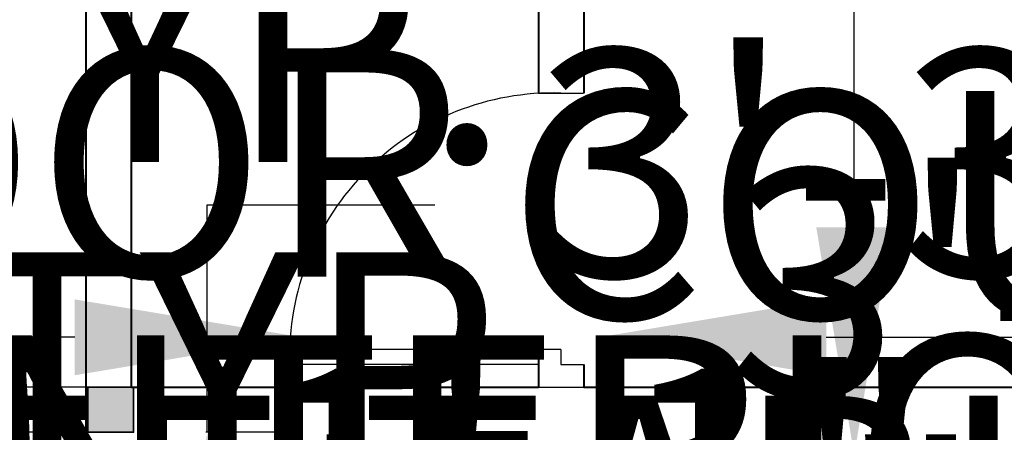
# Model space of a CAD drawing. Units: inches. Extents: x 7323 to 9737, y 2037 to 3322.
# Tile 11 of 19: x 8999 to 9130, y 2513 to 2568. Entities that reach past the tile are written whole.
import ezdxf

# ---------------------------------------------------------------- set-up
doc = ezdxf.new("R2010")
doc.units = ezdxf.units.IN
doc.header["$MEASUREMENT"] = 0
for name, color, linetype, lineweight in [('A-ANNO-DIMS', 2, 'Continuous', 18), ('A-COLS', 1, 'Continuous', 35), ('A-DOOR', 4, 'Continuous', 25), ('A-WALL', 7, 'Continuous', 40)]:
    doc.layers.add(name, color=color, linetype=linetype, lineweight=lineweight)
doc.layers.add('A-COLS-PATT', color=18, linetype='Continuous', lineweight=13, true_color=0x000000)
doc.styles.get("Standard").update_dxf_attribs({"font": 'arial.ttf'})
doc.dimstyles.get("Standard").update_dxf_attribs({"dimtxt": 30.18, "dimasz": 30.18, "dimexe": 0.18, "dimexo": 0.0625, "dimgap": 0.09, "dimtad": 0, "dimtih": 1, "dimtoh": 1, "dimdec": 0, "dimzin": 0, "dimdsep": 46, "dimlunit": 3, "dimtxsty": 'Standard', "dimcen": 0.09, "dimadec": 0, "dimazin": 0, "dimtfac": 1, "dimtdec": 0, "dimtofl": 0, "dimtmove": 0, "dimatfit": 3, "dimfxl": 1, "dimtolj": 1, "dimtzin": 0, "dimarcsym": 0})

# ---------------------------------------------------------------- blocks, each defined once
blk = doc.blocks.new('*D11')
at = {"layer": 'A-ANNO-DIMS', "color": 0, "lineweight": -2, "transparency": 16777216}
for p, q in [((9007.88, 2687.3), (8985.8, 2687.3)), ((8985.98, 2657.12), (8985.98, 2458.79)), ((8985.98, 2229.48), (8985.98, 2427.8)), ((9007.88, 2199.3), (8985.8, 2199.3))]:
    blk.add_line(p, q, dxfattribs=at)
at = {"layer": 'A-ANNO-DIMS', "color": 0, "transparency": 16777216}
for points in [[(8980.95, 2657.12), (8991.01, 2657.12), (8985.98, 2687.3)], [(8980.95, 2229.48), (8991.01, 2229.48), (8985.98, 2199.3)]]:
    blk.add_solid(points, dxfattribs=at)
at = {"layer": 'Defpoints', "color": 0, "transparency": 16777216}
for p in [(9007.95, 2687.3), (8985.98, 2199.3), (9007.95, 2199.3)]:
    blk.add_point(p, dxfattribs=at)
at = {"layer": 'A-ANNO-DIMS', "color": 0, "transparency": 16777216, "insert": (8985.98, 2443.3), "char_height": 30.18, "attachment_point": 5}
blk.add_mtext('\\A1;40\'-8"', dxfattribs=at)
blk = doc.blocks.new('DOOR-36')
for p, q in [((33.01, 39), (39.01, 39)), ((36.01, 5), (0.01, 5)), ((36.01, 5), (36.01, 3)), ((33.01, 3), (0.01, 3)), ((36.01, 3), (39.01, 3)), ((33.01, 0), (39.01, 0))]:
    blk.add_line(p, q)
blk.add_arc((35.01, 4), 35.01, 88.3634, 181.6366)
blk = doc.blocks.new('COL-PLAN-6IN')
blk.add_lwpolyline([(0, 6), (0, 6), (6.06, 6), (6.06, 6), (6.06, 0), (6.06, 0), (0, 0), (0, 0)], close=True)
blk = doc.blocks.new('*D37')
at = {"layer": 'A-ANNO-DIMS', "color": 0, "lineweight": -2, "transparency": 16777216}
for p, q in [((9279.75, 2656.48), (9279.75, 2686.66)), ((9272.01, 2626.3), (9279.93, 2626.3)), ((9272.01, 2574.3), (9279.93, 2574.3)), ((9279.75, 2544.12), (9279.75, 2513.94))]:
    blk.add_line(p, q, dxfattribs=at)
at = {"layer": 'A-ANNO-DIMS', "color": 0, "transparency": 16777216}
for points in [[(9274.72, 2656.48), (9284.78, 2656.48), (9279.75, 2626.3)], [(9274.72, 2544.12), (9284.78, 2544.12), (9279.75, 2574.3)]]:
    blk.add_solid(points, dxfattribs=at)
at = {"layer": 'Defpoints', "color": 0, "transparency": 16777216}
for p in [(9271.95, 2626.3), (9271.95, 2574.3), (9279.75, 2574.3)]:
    blk.add_point(p, dxfattribs=at)
at = {"layer": 'A-ANNO-DIMS', "color": 0, "transparency": 16777216, "insert": (9279.75, 2600.3), "char_height": 30.18, "attachment_point": 5}
blk.add_mtext('\\A1;WINDOW 4\'-4" TYP.', dxfattribs=at)
blk = doc.blocks.new('*D39')
at = {"layer": 'A-ANNO-DIMS', "color": 0, "lineweight": -2, "transparency": 16777216}
for p, q in [((8647.94, 2549.03), (8617.76, 2549.03)), ((8678.12, 2543.2), (8678.12, 2549.21)), ((8717.39, 2543.2), (8717.39, 2549.21)), ((8747.57, 2549.03), (8777.75, 2549.03))]:
    blk.add_line(p, q, dxfattribs=at)
at = {"layer": 'A-ANNO-DIMS', "color": 0, "transparency": 16777216}
for points in [[(8647.94, 2554.06), (8647.94, 2544), (8678.12, 2549.03)], [(8747.57, 2554.06), (8747.57, 2544), (8717.39, 2549.03)]]:
    blk.add_solid(points, dxfattribs=at)
at = {"layer": 'Defpoints', "color": 0, "transparency": 16777216}
for p in [(8717.39, 2549.03), (8678.12, 2543.14), (8717.39, 2543.14)]:
    blk.add_point(p, dxfattribs=at)
at = {"layer": 'A-ANNO-DIMS', "color": 0, "transparency": 16777216, "insert": (9057.19, 2549.03), "char_height": 30.18, "attachment_point": 5}
blk.add_mtext('\\A1;SINGLE DOOR 3\'-3 1/2" TYP.', dxfattribs=at)
blk = doc.blocks.new('*D41')
at = {"layer": 'A-ANNO-DIMS', "color": 0, "lineweight": -2, "transparency": 16777216}
for p, q in [((8661.59, 2428.04), (8661.59, 2458.22)), ((8661.59, 2458.22), (8691.77, 2458.22)), ((8657.46, 2397.86), (8661.77, 2397.86)), ((8657.46, 2369.86), (8661.77, 2369.86)), ((8661.59, 2339.68), (8661.59, 2309.5))]:
    blk.add_line(p, q, dxfattribs=at)
at = {"layer": 'A-ANNO-DIMS', "color": 0, "transparency": 16777216}
for points in [[(8656.56, 2428.04), (8666.62, 2428.04), (8661.59, 2397.86)], [(8656.56, 2339.68), (8666.62, 2339.68), (8661.59, 2369.86)]]:
    blk.add_solid(points, dxfattribs=at)
at = {"layer": 'Defpoints', "color": 0, "transparency": 16777216}
for p in [(8657.39, 2397.86), (8661.59, 2397.86), (8657.39, 2369.86)]:
    blk.add_point(p, dxfattribs=at)
at = {"layer": 'A-ANNO-DIMS', "color": 0, "transparency": 16777216, "insert": (8945.06, 2458.22), "char_height": 30.18, "attachment_point": 5}
blk.add_mtext('\\A1;VENT WINDOW 2\'-4" TYP.', dxfattribs=at)
blk = doc.blocks.new('*D47')
at = {"layer": 'A-ANNO-DIMS', "color": 0, "lineweight": -2, "transparency": 16777216}
for p, q in [((8839.73, 2461.79), (8839.73, 2464.67)), ((8858.14, 2461.79), (8858.14, 2464.67)), ((8809.55, 2464.49), (8779.37, 2464.49)), ((8888.32, 2464.49), (8918.5, 2464.49))]:
    blk.add_line(p, q, dxfattribs=at)
at = {"layer": 'A-ANNO-DIMS', "color": 0, "transparency": 16777216}
for points in [[(8809.55, 2469.52), (8809.55, 2459.46), (8839.73, 2464.49)], [(8888.32, 2469.52), (8888.32, 2459.46), (8858.14, 2464.49)]]:
    blk.add_solid(points, dxfattribs=at)
at = {"layer": 'Defpoints', "color": 0, "transparency": 16777216}
for p in [(8858.14, 2464.49), (8839.73, 2461.73), (8858.14, 2461.73)]:
    blk.add_point(p, dxfattribs=at)
at = {"layer": 'A-ANNO-DIMS', "color": 0, "transparency": 16777216, "insert": (9164.9, 2464.49), "char_height": 30.18, "attachment_point": 5}
blk.add_mtext('\\A1;ARMCHAIR 1\'-6 1/2" TYP.', dxfattribs=at)
blk = doc.blocks.new('*D48')
at = {"layer": 'A-ANNO-DIMS', "color": 0, "lineweight": -2, "transparency": 16777216}
for p, q in [((8836.96, 2491.91), (8836.96, 2522.09)), ((8836.96, 2522.09), (8867.14, 2522.09)), ((8839.66, 2461.73), (8836.78, 2461.73)), ((8839.66, 2451.75), (8836.78, 2451.75)), ((8836.96, 2421.57), (8836.96, 2391.39))]:
    blk.add_line(p, q, dxfattribs=at)
at = {"layer": 'A-ANNO-DIMS', "color": 0, "transparency": 16777216}
for points in [[(8831.93, 2491.91), (8841.99, 2491.91), (8836.96, 2461.73)], [(8831.93, 2421.57), (8841.99, 2421.57), (8836.96, 2451.75)]]:
    blk.add_solid(points, dxfattribs=at)
at = {"layer": 'Defpoints', "color": 0, "transparency": 16777216}
for p in [(8836.96, 2461.73), (8839.73, 2461.73), (8839.73, 2451.75)]:
    blk.add_point(p, dxfattribs=at)
at = {"layer": 'A-ANNO-DIMS', "color": 0, "transparency": 16777216, "insert": (8970.94, 2522.09), "char_height": 30.18, "attachment_point": 5}
blk.add_mtext('\\A1;0\'-10" TYP.', dxfattribs=at)
blk = doc.blocks.new('*D52')
at = {"layer": 'A-ANNO-DIMS', "color": 0, "lineweight": -2, "transparency": 16777216}
for p, q in [((9220.65, 2583.03), (9220.65, 2613.21)), ((9209.01, 2552.85), (9220.83, 2552.85)), ((9209.01, 2513.3), (9220.83, 2513.3)), ((9220.65, 2483.12), (9220.65, 2452.94))]:
    blk.add_line(p, q, dxfattribs=at)
at = {"layer": 'A-ANNO-DIMS', "color": 0, "transparency": 16777216}
for points in [[(9215.62, 2583.03), (9225.68, 2583.03), (9220.65, 2552.85)], [(9215.62, 2483.12), (9225.68, 2483.12), (9220.65, 2513.3)]]:
    blk.add_solid(points, dxfattribs=at)
at = {"layer": 'Defpoints', "color": 0, "transparency": 16777216}
for p in [(9208.95, 2552.85), (9220.65, 2552.85), (9208.95, 2513.3)]:
    blk.add_point(p, dxfattribs=at)
at = {"layer": 'A-ANNO-DIMS', "color": 0, "transparency": 16777216, "insert": (9220.65, 2533.07), "char_height": 30.18, "attachment_point": 5}
blk.add_mtext('\\A1;3\'-3 1/2" TYP.', dxfattribs=at)
blk = doc.blocks.new('*D53')
at = {"layer": 'A-ANNO-DIMS', "color": 0, "lineweight": -2, "transparency": 16777216}
for p, q in [((8826.85, 2511.06), (8796.67, 2511.06)), ((8857.03, 2503.93), (8857.03, 2511.24)), ((8905.03, 2503.93), (8905.03, 2511.24)), ((8935.21, 2511.06), (8965.39, 2511.06))]:
    blk.add_line(p, q, dxfattribs=at)
at = {"layer": 'A-ANNO-DIMS', "color": 0, "transparency": 16777216}
for points in [[(8826.85, 2516.09), (8826.85, 2506.03), (8857.03, 2511.06)], [(8935.21, 2516.09), (8935.21, 2506.03), (8905.03, 2511.06)]]:
    blk.add_solid(points, dxfattribs=at)
at = {"layer": 'Defpoints', "color": 0, "transparency": 16777216}
for p in [(8905.03, 2511.06), (8857.03, 2503.86), (8905.03, 2503.86)]:
    blk.add_point(p, dxfattribs=at)
at = {"layer": 'A-ANNO-DIMS', "color": 0, "transparency": 16777216, "insert": (9261.3, 2511.06), "char_height": 30.18, "attachment_point": 5}
blk.add_mtext('\\A1;INTERIOR WINDOW 4\'-0" TYP.', dxfattribs=at)
blk = doc.blocks.new('*D54')
at = {"layer": 'A-ANNO-DIMS', "color": 0, "lineweight": -2, "transparency": 16777216}
for p, q in [((8849.83, 2534.04), (8849.83, 2564.22)), ((8849.83, 2564.22), (8880.01, 2564.22)), ((8856.96, 2503.86), (8849.65, 2503.86)), ((8856.96, 2497.86), (8849.65, 2497.86)), ((8849.83, 2467.68), (8849.83, 2437.5))]:
    blk.add_line(p, q, dxfattribs=at)
at = {"layer": 'A-ANNO-DIMS', "color": 0, "transparency": 16777216}
for points in [[(8844.8, 2534.04), (8854.86, 2534.04), (8849.83, 2503.86)], [(8844.8, 2467.68), (8854.86, 2467.68), (8849.83, 2497.86)]]:
    blk.add_solid(points, dxfattribs=at)
at = {"layer": 'Defpoints', "color": 0, "transparency": 16777216}
for p in [(8849.83, 2503.86), (8857.03, 2503.86), (8857.03, 2497.86)]:
    blk.add_point(p, dxfattribs=at)
at = {"layer": 'A-ANNO-DIMS', "color": 0, "transparency": 16777216, "insert": (8972.08, 2564.22), "char_height": 30.18, "attachment_point": 5}
blk.add_mtext('\\A1;0\'-6" TYP.', dxfattribs=at)
blk = doc.blocks.new('*D59')
at = {"layer": 'A-ANNO-DIMS', "color": 0, "lineweight": -2, "transparency": 16777216}
for p, q in [((9064.67, 2473.96), (9064.67, 2467.95)), ((9103.95, 2473.96), (9103.95, 2467.95)), ((9034.49, 2468.13), (9004.31, 2468.13)), ((9134.13, 2468.13), (9164.31, 2468.13))]:
    blk.add_line(p, q, dxfattribs=at)
at = {"layer": 'A-ANNO-DIMS', "color": 0, "transparency": 16777216}
for points in [[(9034.49, 2473.16), (9034.49, 2463.1), (9064.67, 2468.13)], [(9134.13, 2473.16), (9134.13, 2463.1), (9103.95, 2468.13)]]:
    blk.add_solid(points, dxfattribs=at)
at = {"layer": 'Defpoints', "color": 0, "transparency": 16777216}
for p in [(9064.67, 2474.02), (9103.95, 2474.02), (9103.95, 2468.13)]:
    blk.add_point(p, dxfattribs=at)
at = {"layer": 'A-ANNO-DIMS', "color": 0, "transparency": 16777216, "insert": (9458.35, 2468.13), "char_height": 30.18, "attachment_point": 5}
blk.add_mtext('\\A1;KITCHEN DOOR 3\'-3 1/2" TYP.', dxfattribs=at)
blk = doc.blocks.new('*D60')
at = {"layer": 'A-ANNO-DIMS', "color": 0, "lineweight": -2, "transparency": 16777216}
for p, q in [((9109.84, 2540.48), (9109.84, 2570.66)), ((9104.01, 2510.3), (9110.02, 2510.3)), ((9104.01, 2474.02), (9110.02, 2474.02)), ((9109.84, 2443.84), (9109.84, 2413.66))]:
    blk.add_line(p, q, dxfattribs=at)
at = {"layer": 'A-ANNO-DIMS', "color": 0, "transparency": 16777216}
for points in [[(9104.81, 2540.48), (9114.87, 2540.48), (9109.84, 2510.3)], [(9104.81, 2443.84), (9114.87, 2443.84), (9109.84, 2474.02)]]:
    blk.add_solid(points, dxfattribs=at)
at = {"layer": 'Defpoints', "color": 0, "transparency": 16777216}
for p in [(9103.95, 2510.3), (9109.84, 2510.3), (9103.95, 2474.02)]:
    blk.add_point(p, dxfattribs=at)
at = {"layer": 'A-ANNO-DIMS', "color": 0, "transparency": 16777216, "insert": (9109.84, 2492.16), "char_height": 30.18, "attachment_point": 5}
blk.add_mtext('\\A1;3\'-0 1/2" TYP.', dxfattribs=at)
blk = doc.blocks.new('*D63')
at = {"layer": 'A-ANNO-DIMS', "color": 0, "lineweight": -2, "transparency": 16777216}
for p, q in [((8744.72, 2466.22), (8744.72, 2496.4)), ((8744.72, 2496.4), (8774.9, 2496.4)), ((8741.46, 2436.04), (8744.9, 2436.04)), ((8741.46, 2413.86), (8744.9, 2413.86)), ((8744.72, 2383.68), (8744.72, 2353.5))]:
    blk.add_line(p, q, dxfattribs=at)
at = {"layer": 'A-ANNO-DIMS', "color": 0, "transparency": 16777216}
for points in [[(8739.69, 2466.22), (8749.75, 2466.22), (8744.72, 2436.04)], [(8739.69, 2383.68), (8749.75, 2383.68), (8744.72, 2413.86)]]:
    blk.add_solid(points, dxfattribs=at)
at = {"layer": 'Defpoints', "color": 0, "transparency": 16777216}
for p in [(8741.39, 2436.04), (8744.72, 2436.04), (8741.39, 2413.86)]:
    blk.add_point(p, dxfattribs=at)
at = {"layer": 'A-ANNO-DIMS', "color": 0, "transparency": 16777216, "insert": (9003.76, 2496.4), "char_height": 30.18, "attachment_point": 5}
blk.add_mtext('\\A1;APPLIANCE 1\'-10" TYP.', dxfattribs=at)
blk = doc.blocks.new('*D65')
at = {"layer": 'A-ANNO-DIMS', "color": 0, "lineweight": -2, "transparency": 16777216}
for p, q in [((9024.02, 2513.3), (9024.02, 2543.48)), ((9024.02, 2543.48), (9054.2, 2543.48)), ((9036.56, 2513.3), (9023.84, 2513.3)), ((9024.02, 2459.48), (9024.02, 2483.12)), ((9036.56, 2429.3), (9023.84, 2429.3))]:
    blk.add_line(p, q, dxfattribs=at)
at = {"layer": 'A-ANNO-DIMS', "color": 0, "transparency": 16777216}
for points in [[(9018.99, 2483.12), (9029.05, 2483.12), (9024.02, 2513.3)], [(9018.99, 2459.48), (9029.05, 2459.48), (9024.02, 2429.3)]]:
    blk.add_solid(points, dxfattribs=at)
at = {"layer": 'Defpoints', "color": 0, "transparency": 16777216}
for p in [(9024.02, 2513.3), (9036.62, 2513.3), (9036.62, 2429.3)]:
    blk.add_point(p, dxfattribs=at)
at = {"layer": 'A-ANNO-DIMS', "color": 0, "transparency": 16777216, "insert": (9256.18, 2543.48), "char_height": 30.18, "attachment_point": 5}
blk.add_mtext('\\A1;COUNTER 7\'-0" TYP.', dxfattribs=at)
blk = doc.blocks.new('*D66')
at = {"layer": 'A-ANNO-DIMS', "color": 0, "lineweight": -2, "transparency": 16777216}
for p, q in [((9036.62, 2513.36), (9036.62, 2526.08)), ((9075.95, 2513.36), (9075.95, 2526.08)), ((9006.44, 2525.9), (8976.26, 2525.9)), ((9106.13, 2525.9), (9136.31, 2525.9))]:
    blk.add_line(p, q, dxfattribs=at)
at = {"layer": 'A-ANNO-DIMS', "color": 0, "transparency": 16777216}
for points in [[(9006.44, 2530.93), (9006.44, 2520.87), (9036.62, 2525.9)], [(9106.13, 2530.93), (9106.13, 2520.87), (9075.95, 2525.9)]]:
    blk.add_solid(points, dxfattribs=at)
at = {"layer": 'Defpoints', "color": 0, "transparency": 16777216}
for p in [(9075.95, 2525.9), (9036.62, 2513.3), (9075.95, 2513.3)]:
    blk.add_point(p, dxfattribs=at)
at = {"layer": 'A-ANNO-DIMS', "color": 0, "transparency": 16777216, "insert": (9263.53, 2525.9), "char_height": 30.18, "attachment_point": 5}
blk.add_mtext('\\A1;3\'-3 1/2" TYP.', dxfattribs=at)
blk = doc.blocks.new('*D69')
at = {"layer": 'A-ANNO-DIMS', "color": 0, "lineweight": -2, "transparency": 16777216}
for p, q in [((8836.58, 2472.89), (8836.58, 2503.07)), ((8836.58, 2503.07), (8866.76, 2503.07)), ((8839.88, 2442.71), (8836.4, 2442.71)), ((8839.88, 2420.33), (8836.4, 2420.33)), ((8836.58, 2390.15), (8836.58, 2359.97))]:
    blk.add_line(p, q, dxfattribs=at)
at = {"layer": 'A-ANNO-DIMS', "color": 0, "transparency": 16777216}
for points in [[(8831.55, 2472.89), (8841.61, 2472.89), (8836.58, 2442.71)], [(8831.55, 2390.15), (8841.61, 2390.15), (8836.58, 2420.33)]]:
    blk.add_solid(points, dxfattribs=at)
at = {"layer": 'Defpoints', "color": 0, "transparency": 16777216}
for p in [(8836.58, 2442.71), (8839.94, 2442.71), (8839.94, 2420.33)]:
    blk.add_point(p, dxfattribs=at)
at = {"layer": 'A-ANNO-DIMS', "color": 0, "transparency": 16777216, "insert": (9169.54, 2503.07), "char_height": 30.18, "attachment_point": 5}
blk.add_mtext('\\A1;COFFEE TABLE 1\'-10 1/2" TYP.', dxfattribs=at)
blk = doc.blocks.new('*D71')
at = {"layer": 'A-ANNO-DIMS', "color": 0, "lineweight": -2, "transparency": 16777216}
for p, q in [((8891.18, 2486.02), (8891.18, 2516.2)), ((8884.24, 2455.84), (8891.36, 2455.84)), ((8884.24, 2409.18), (8891.36, 2409.18)), ((8891.18, 2379), (8891.18, 2348.82))]:
    blk.add_line(p, q, dxfattribs=at)
at = {"layer": 'A-ANNO-DIMS', "color": 0, "transparency": 16777216}
for points in [[(8886.15, 2486.02), (8896.21, 2486.02), (8891.18, 2455.84)], [(8886.15, 2379), (8896.21, 2379), (8891.18, 2409.18)]]:
    blk.add_solid(points, dxfattribs=at)
at = {"layer": 'Defpoints', "color": 0, "transparency": 16777216}
for p in [(8884.18, 2455.84), (8891.18, 2455.84), (8884.18, 2409.18)]:
    blk.add_point(p, dxfattribs=at)
at = {"layer": 'A-ANNO-DIMS', "color": 0, "transparency": 16777216, "insert": (8891.18, 2432.51), "char_height": 30.18, "attachment_point": 5}
blk.add_mtext('\\A1;SOFA 3\'-10 1/2" TYP.', dxfattribs=at)
blk = doc.blocks.new('*D74')
at = {"layer": 'A-ANNO-DIMS', "color": 0, "lineweight": -2, "transparency": 16777216}
for p, q in [((9059.91, 2453.48), (9059.91, 2483.66)), ((9059.91, 2483.66), (9090.09, 2483.66)), ((9061.53, 2423.3), (9059.73, 2423.3)), ((9061.53, 2413.24), (9059.73, 2413.24)), ((9059.91, 2383.06), (9059.91, 2352.88))]:
    blk.add_line(p, q, dxfattribs=at)
at = {"layer": 'A-ANNO-DIMS', "color": 0, "transparency": 16777216}
for points in [[(9054.88, 2453.48), (9064.94, 2453.48), (9059.91, 2423.3)], [(9054.88, 2383.06), (9064.94, 2383.06), (9059.91, 2413.24)]]:
    blk.add_solid(points, dxfattribs=at)
at = {"layer": 'Defpoints', "color": 0, "transparency": 16777216}
for p in [(9059.91, 2423.3), (9061.59, 2423.3), (9061.59, 2413.24)]:
    blk.add_point(p, dxfattribs=at)
at = {"layer": 'A-ANNO-DIMS', "color": 0, "transparency": 16777216, "insert": (9193.89, 2483.66), "char_height": 30.18, "attachment_point": 5}
blk.add_mtext('\\A1;0\'-10" TYP.', dxfattribs=at)
blk = doc.blocks.new('*D79')
at = {"layer": 'A-ANNO-DIMS', "color": 0, "lineweight": -2, "transparency": 16777216}
for p, q in [((8871.1, 2395.97), (8871.1, 2394.46)), ((8880.36, 2395.97), (8880.36, 2394.46)), ((8840.92, 2394.64), (8810.74, 2394.64)), ((8910.54, 2394.64), (8940.72, 2394.64))]:
    blk.add_line(p, q, dxfattribs=at)
at = {"layer": 'A-ANNO-DIMS', "color": 0, "transparency": 16777216}
for points in [[(8840.92, 2399.67), (8840.92, 2389.61), (8871.1, 2394.64)], [(8910.54, 2399.67), (8910.54, 2389.61), (8880.36, 2394.64)]]:
    blk.add_solid(points, dxfattribs=at)
at = {"layer": 'Defpoints', "color": 0, "transparency": 16777216}
for p in [(8871.1, 2396.03), (8880.36, 2396.03), (8880.36, 2394.64)]:
    blk.add_point(p, dxfattribs=at)
at = {"layer": 'A-ANNO-DIMS', "color": 0, "transparency": 16777216, "insert": (9195.57, 2394.64), "char_height": 30.18, "attachment_point": 5}
blk.add_mtext('\\A1;SIDE TABLE 0\'-9 1/2" TYP.', dxfattribs=at)
blk = doc.blocks.new('*D100')
at = {"layer": 'A-ANNO-DIMS', "color": 0, "lineweight": -2, "transparency": 16777216}
for p, q in [((9007.88, 2687.3), (8587.16, 2687.3)), ((8587.34, 2657.12), (8587.34, 2615.8)), ((8587.34, 2543.49), (8587.34, 2584.8)), ((9008.12, 2513.31), (8587.16, 2513.31))]:
    blk.add_line(p, q, dxfattribs=at)
at = {"layer": 'A-ANNO-DIMS', "color": 0, "transparency": 16777216}
for points in [[(8582.31, 2657.12), (8592.37, 2657.12), (8587.34, 2687.3)], [(8582.31, 2543.49), (8592.37, 2543.49), (8587.34, 2513.31)]]:
    blk.add_solid(points, dxfattribs=at)
at = {"layer": 'Defpoints', "color": 0, "transparency": 16777216}
for p in [(9007.95, 2687.3), (8587.34, 2513.31), (9008.18, 2513.31)]:
    blk.add_point(p, dxfattribs=at)
at = {"layer": 'A-ANNO-DIMS', "color": 0, "transparency": 16777216, "insert": (8587.34, 2600.3), "char_height": 30.18, "attachment_point": 5}
blk.add_mtext('\\A1;14\'-6"', dxfattribs=at)
blk = doc.blocks.new('*D106')
at = {"layer": 'A-ANNO-DIMS', "color": 0, "lineweight": -2, "transparency": 16777216}
for p, q in [((9008.12, 2519.31), (8587.16, 2519.31)), ((8587.34, 2489.13), (8587.34, 2439.14)), ((8587.34, 2357.76), (8587.34, 2407.75)), ((9008.23, 2327.58), (8587.16, 2327.58))]:
    blk.add_line(p, q, dxfattribs=at)
at = {"layer": 'A-ANNO-DIMS', "color": 0, "transparency": 16777216}
for points in [[(8582.31, 2489.13), (8592.37, 2489.13), (8587.34, 2519.31)], [(8582.31, 2357.76), (8592.37, 2357.76), (8587.34, 2327.58)]]:
    blk.add_solid(points, dxfattribs=at)
at = {"layer": 'Defpoints', "color": 0, "transparency": 16777216}
for p in [(8587.34, 2519.31), (9008.18, 2519.31), (9008.29, 2327.58)]:
    blk.add_point(p, dxfattribs=at)
at = {"layer": 'A-ANNO-DIMS', "color": 0, "transparency": 16777216, "insert": (8587.34, 2423.44), "char_height": 30.18, "attachment_point": 5}
blk.add_mtext('\\A1;15\'-11 1/2"', dxfattribs=at)
blk = doc.blocks.new('*D112')
at = {"layer": 'A-ANNO-DIMS', "color": 0, "lineweight": -2, "transparency": 16777216}
for p, q in [((9006.28, 2476.47), (9006.28, 2506.65)), ((9006.28, 2506.65), (9036.46, 2506.65)), ((9041.42, 2446.29), (9006.1, 2446.29)), ((9041.42, 2433.19), (9006.1, 2433.19)), ((9006.28, 2403.01), (9006.28, 2372.83))]:
    blk.add_line(p, q, dxfattribs=at)
at = {"layer": 'A-ANNO-DIMS', "color": 0, "transparency": 16777216}
for points in [[(9001.25, 2476.47), (9011.31, 2476.47), (9006.28, 2446.29)], [(9001.25, 2403.01), (9011.31, 2403.01), (9006.28, 2433.19)]]:
    blk.add_solid(points, dxfattribs=at)
at = {"layer": 'Defpoints', "color": 0, "transparency": 16777216}
for p in [(9006.28, 2446.29), (9041.48, 2446.29), (9041.48, 2433.19)]:
    blk.add_point(p, dxfattribs=at)
at = {"layer": 'A-ANNO-DIMS', "color": 0, "transparency": 16777216, "insert": (9075.24, 2506.65), "char_height": 30.18, "attachment_point": 5}
blk.add_mtext('\\A1;1\'-1"', dxfattribs=at)
blk = doc.blocks.new('*D114')
at = {"layer": 'A-ANNO-DIMS', "color": 0, "lineweight": -2, "transparency": 16777216}
for p, q in [((8915.46, 2671.86), (9307.45, 2671.86)), ((9307.27, 2641.68), (9307.27, 2641.04)), ((8915.46, 2610.86), (9307.45, 2610.86)), ((9307.27, 2610.86), (9307.27, 2580.68)), ((9307.27, 2580.68), (9277.09, 2580.68))]:
    blk.add_line(p, q, dxfattribs=at)
at = {"layer": 'A-ANNO-DIMS', "color": 0, "transparency": 16777216}
for points in [[(9302.24, 2641.68), (9312.3, 2641.68), (9307.27, 2671.86)], [(9302.24, 2641.04), (9312.3, 2641.04), (9307.27, 2610.86)]]:
    blk.add_solid(points, dxfattribs=at)
at = {"layer": 'Defpoints', "color": 0, "transparency": 16777216}
for p in [(8915.39, 2671.86), (8915.39, 2610.86), (9307.27, 2610.86)]:
    blk.add_point(p, dxfattribs=at)
at = {"layer": 'A-ANNO-DIMS', "color": 0, "transparency": 16777216, "insert": (9236.89, 2580.68), "char_height": 30.18, "attachment_point": 5}
blk.add_mtext('\\A1;5\'-1"', dxfattribs=at)
blk = doc.blocks.new('*D126')
at = {"layer": 'A-ANNO-DIMS', "color": 0, "lineweight": -2, "transparency": 16777216}
for p, q in [((9109.28, 2586.63), (9139.46, 2586.63)), ((9139.46, 2586.63), (9160.18, 2564.69)), ((9204.86, 2517.3), (9205.04, 2517.3)), ((9204.95, 2517.21), (9204.95, 2517.39))]:
    blk.add_line(p, q, dxfattribs=at)
at = {"layer": 'A-ANNO-DIMS', "color": 0, "transparency": 16777216}
blk.add_solid([(9163.84, 2568.15), (9156.52, 2561.24), (9180.9, 2542.75)], dxfattribs=at)
at = {"layer": 'Defpoints', "color": 0, "transparency": 16777216}
for p in [(9180.9, 2542.75), (9204.95, 2517.3)]:
    blk.add_point(p, dxfattribs=at)
at = {"layer": 'A-ANNO-DIMS', "color": 0, "transparency": 16777216, "insert": (9009.88, 2586.63), "char_height": 30.18, "attachment_point": 5}
blk.add_mtext('\\A1;4X R2\'-11"', dxfattribs=at)

msp = doc.modelspace()

# ---------------------------------------------------------------- hatches: boundary and pattern name
at = {"layer": 'A-COLS-PATT'}
h = msp.add_hatch(color=256, dxfattribs=at)
h.dxf.hatch_style = 1
h.paths.add_polyline_path([(8915.39, 2189.86), (8908.77, 2189.86), (8908.77, 2183.86), (8915.39, 2183.86)])
h.paths.add_polyline_path([(8657.61, 2189.86), (8651.55, 2189.86), (8651.55, 2183.86), (8657.61, 2183.86)])
h.paths.add_polyline_path([(8814.13, 2189.86), (8807.39, 2189.86), (8807.39, 2183.86), (8814.13, 2183.86)])
h.paths.add_polyline_path([(8813.39, 2317.86), (8807.36, 2317.86), (8807.36, 2311.86), (8813.39, 2311.86)])
h.paths.add_polyline_path([(8915.34, 2313.13), (8909.39, 2313.13), (8909.39, 2307.13), (8915.34, 2307.13)])
h.paths.add_polyline_path([(8657.62, 2317.86), (8657.39, 2317.86), (8657.39, 2318.08), (8651.55, 2318.08), (8651.55, 2312.08), (8657.62, 2312.08)])
h.paths.add_polyline_path([(8915.39, 2671.84), (8909.37, 2671.84), (8909.37, 2665.86), (8909.39, 2665.86), (8915.39, 2665.84)])
h.paths.add_polyline_path([(8657.59, 2671.81), (8651.52, 2671.81), (8651.52, 2665.81), (8657.39, 2665.81), (8657.39, 2665.86)])
h.paths.add_polyline_path([(8915.28, 2503.94), (8909.39, 2503.94), (8909.39, 2503.86), (8909.22, 2497.94), (8915.28, 2497.94)])
h.paths.add_polyline_path([(8657.53, 2503.86), (8657.39, 2503.86), (8651.46, 2503.96), (8651.46, 2497.96), (8657.53, 2497.96)])
h.paths.add_polyline_path([(9014.24, 2519.3), (9013.95, 2519.3), (9008.18, 2519.31), (9008.18, 2513.31), (9014.24, 2513.31)])
h.paths.add_polyline_path([(9013.95, 2687.3), (9007.95, 2687.3), (9007.95, 2681.3), (9013.95, 2681.3)])
h.paths.add_polyline_path([(9271.95, 2687.3), (9266.01, 2687.3), (9266.01, 2681.35), (9271.95, 2681.35)])
h.paths.add_polyline_path([(9271.95, 2205.3), (9265.32, 2205.3), (9265.32, 2199.3), (9271.95, 2199.3)])
h.paths.add_polyline_path([(9170.68, 2205.3), (9163.95, 2205.3), (9163.95, 2199.3), (9170.68, 2199.3)])
h.paths.add_polyline_path([(9013.95, 2205.3), (9007.95, 2205.3), (9007.95, 2199.3), (9013.95, 2199.3)])
h.paths.add_polyline_path([(9271.95, 2519.51), (9265.95, 2519.51), (9265.95, 2519.3), (9265.93, 2513.51), (9271.95, 2513.51)])
h.paths.add_polyline_path([(9271.95, 2328.64), (9265.95, 2328.64), (9265.95, 2322.64), (9271.95, 2322.64)])
h.paths.add_polyline_path([(9014.35, 2333.3), (9013.95, 2333.3), (9013.95, 2333.58), (9008.29, 2333.58), (9008.29, 2327.58), (9014.35, 2327.58)])

# ---------------------------------------------------------------- linework, layer by layer
at = {"layer": 'A-WALL'}
for p, q in [((9007.95, 2199.3), (9007.95, 2687.3)), ((9013.95, 2519.3), (9013.95, 2681.3)), ((9067.95, 2681.3), (9067.95, 2558.25)), ((9073.95, 2681.3), (9073.95, 2558.3)), ((9067.95, 2524.3), (9067.95, 2519.3)), ((9073.95, 2522.3), (9073.95, 2519.3)), ((9013.95, 2519.3), (9067.95, 2519.3)), ((9073.95, 2519.3), (9135.95, 2519.3))]:
    msp.add_line(p, q, dxfattribs=at)

# ---------------------------------------------------------------- block references
at = {"layer": 'A-COLS'}
msp.add_blockref('COL-PLAN-6IN', (9008.18, 2513.31), dxfattribs=at)
at = {"layer": 'A-DOOR'}
msp.add_blockref('DOOR-36', (9034.93, 2519.3), dxfattribs=at)

# ---------------------------------------------------------------- dimensions: what is measured, and where the dimension line sits
at = {"layer": 'A-ANNO-DIMS'}
for base, p1, p2, override, picture, middle in [((8587.34, 2513.31), (9007.95, 2687.3), (9008.18, 2513.31), {"dimdec": 1, "dimlfac": 1, "dimrnd": 0, "dimzin": 1, "dimdsep": 46, "dimlunit": 4, "dimfrac": 2}, '*D100', (8587.34, 2600.3)), ((8985.98, 2199.3), (9007.95, 2687.3), (9007.95, 2199.3), {"dimclrd": 0, "dimclre": 0, "dimclrt": 0}, '*D11', (8985.98, 2443.3)), ((9307.27, 2610.86), (8915.39, 2671.86), (8915.39, 2610.86), {"dimdec": 1, "dimlfac": 1, "dimrnd": 0, "dimzin": 1, "dimdsep": 46, "dimlunit": 4, "dimfrac": 2}, '*D114', (9236.89, 2580.68)), ((9006.28, 2446.29), (9041.48, 2433.19), (9041.48, 2446.29), {"dimdec": 1, "dimlfac": 1, "dimrnd": 0, "dimzin": 1, "dimdsep": 46, "dimlunit": 4, "dimfrac": 2}, '*D112', (9075.24, 2506.65)), ((8587.34, 2519.31), (9008.29, 2327.58), (9008.18, 2519.31), {"dimdec": 1, "dimlfac": 1, "dimrnd": 0, "dimzin": 1, "dimdsep": 46, "dimlunit": 4, "dimfrac": 2}, '*D106', (8587.34, 2423.44))]:
    dim = msp.add_linear_dim(base=base, p1=p1, p2=p2, angle=90, dimstyle='Standard', override=override, dxfattribs=at)
    dim.commit()
    dim.dimension.update_dxf_attribs({"geometry": picture, "text_midpoint": middle})
for base, p1, p2, angle, text, picture, middle in [((9279.75, 2574.3), (9271.95, 2626.3), (9271.95, 2574.3), 270, 'WINDOW <> TYP.', '*D37', (9279.75, 2600.3)), ((8836.58, 2442.71), (8839.94, 2420.33), (8839.94, 2442.71), 90, 'COFFEE TABLE <> TYP.', '*D69', (9169.54, 2503.07)), ((9024.02, 2513.3), (9036.62, 2429.3), (9036.62, 2513.3), 90, 'COUNTER <> TYP.', '*D65', (9256.18, 2543.48)), ((9220.6454, 2552.8475), (9208.9454, 2513.2952), (9208.9454, 2552.8475), 90, '<> TYP.', '*D52', (9220.6454, 2533.0713)), ((8849.83, 2503.86), (8857.03, 2497.86), (8857.03, 2503.86), 90, '<> TYP.', '*D54', (8972.08, 2564.22)), ((9109.84, 2510.3), (9103.95, 2474.02), (9103.95, 2510.3), 90, '<> TYP.', '*D60', (9109.84, 2492.16)), ((8744.72, 2436.04), (8741.39, 2413.86), (8741.39, 2436.04), 90, 'APPLIANCE <> TYP.', '*D63', (9003.76, 2496.4)), ((8836.96, 2461.73), (8839.73, 2451.75), (8839.73, 2461.73), 90, '<> TYP.', '*D48', (8970.94, 2522.09)), ((8661.59, 2397.86), (8657.39, 2369.86), (8657.39, 2397.86), 90, 'VENT WINDOW <> TYP.', '*D41', (8945.06, 2458.22)), ((9059.91, 2423.3), (9061.59, 2413.24), (9061.59, 2423.3), 90, '<> TYP.', '*D74', (9193.89, 2483.66)), ((8891.18, 2455.84), (8884.18, 2409.18), (8884.18, 2455.84), 90, 'SOFA <> TYP.', '*D71', (8891.18, 2432.51))]:
    dim = msp.add_linear_dim(base=base, p1=p1, p2=p2, angle=angle, text=text, dimstyle='Standard', override={"dimdec": 1, "dimlfac": 1, "dimrnd": 0, "dimzin": 1, "dimdsep": 46, "dimlunit": 4, "dimfrac": 2}, dxfattribs=at)
    dim.commit()
    dim.dimension.update_dxf_attribs({"geometry": picture, "text_midpoint": middle})
for base, p1, p2, text, picture, middle in [((8717.39, 2549.03), (8678.12, 2543.14), (8717.39, 2543.14), 'SINGLE DOOR <> TYP.', '*D39', (9057.19, 2549.03)), ((8905.03, 2511.06), (8857.03, 2503.86), (8905.03, 2503.86), 'INTERIOR WINDOW <> TYP.', '*D53', (9261.3, 2511.06)), ((9075.95, 2525.9), (9036.62, 2513.3), (9075.95, 2513.3), '<> TYP.', '*D66', (9263.53, 2525.9)), ((9103.95, 2468.13), (9064.67, 2474.02), (9103.95, 2474.02), 'KITCHEN DOOR <> TYP.', '*D59', (9458.35, 2468.13)), ((8858.14, 2464.49), (8839.73, 2461.73), (8858.14, 2461.73), 'ARMCHAIR <> TYP.', '*D47', (9164.9, 2464.49)), ((8880.36, 2394.64), (8871.1, 2396.03), (8880.36, 2396.03), 'SIDE TABLE <> TYP.', '*D79', (9195.57, 2394.64))]:
    dim = msp.add_linear_dim(base=base, p1=p1, p2=p2, text=text, dimstyle='Standard', override={"dimdec": 1, "dimlfac": 1, "dimrnd": 0, "dimzin": 1, "dimdsep": 46, "dimlunit": 4, "dimfrac": 2}, dxfattribs=at)
    dim.commit()
    dim.dimension.update_dxf_attribs({"geometry": picture, "text_midpoint": middle})
dim = msp.add_radius_dim(center=(9204.95, 2517.3), mpoint=(9180.9, 2542.75), text='4X <>', dimstyle='Standard', override={"dimdec": 1, "dimlfac": 1, "dimrnd": 0, "dimzin": 1, "dimdsep": 46, "dimlunit": 4, "dimfrac": 2}, dxfattribs=at)
dim.commit()
dim.dimension.update_dxf_attribs({"geometry": '*D126', "text_midpoint": (9009.88, 2586.63)})

doc.saveas('drawing.dxf')
